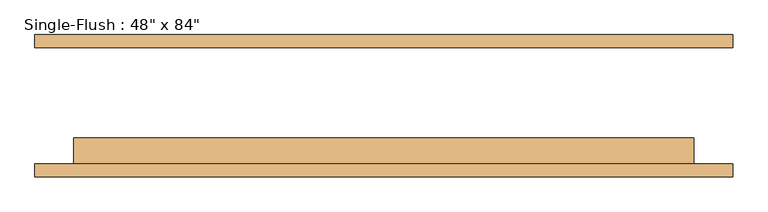
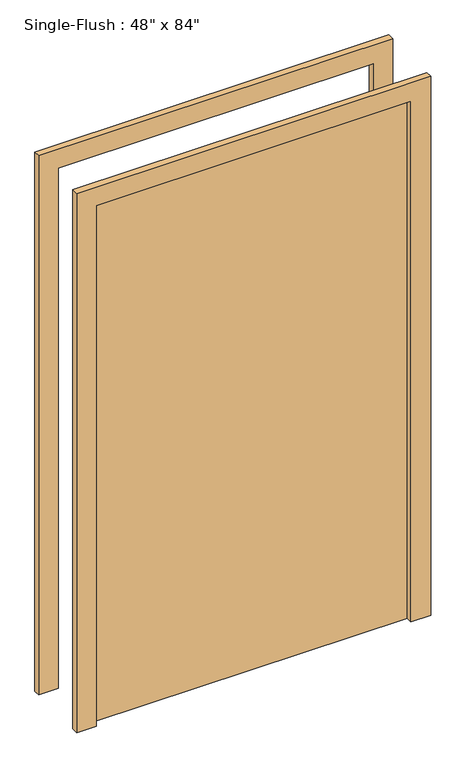
"""IFC4 building model written with IfcOpenShell, lengths in millimetres: door geometry."""

from ifc_helpers import new_model, si_unit, frame, origin, origin_with_axes, place, context, project, spatial, polyline, outline, extrude, source, transform, mapped, element, save


def door_f4c4cdf2(model_context):
    return source(origin(), model_context, "Body", "SweptSolid", [
        extrude(outline(polyline([(2209.8, -685.8), (0.0, -685.8), (0.0, -609.6), (2133.6, -609.6), (2133.6, 609.6), (0.0, 609.6), (0.0, 685.8), (2209.8, 685.8), (2209.8, -685.8)])), frame((0.0, -139.7, 0.0), z_axis=(0.0, 1.0, 0.0), x_axis=(0.0, 0.0, 1.0)), (0.0, 0.0, 1.0), 25.4),
        extrude(outline(polyline([(2209.8, 685.8), (2209.8, -685.8), (0.0, -685.8), (0.0, -609.6), (2133.6, -609.6), (2133.6, 609.6), (0.0, 609.6), (0.0, 685.8), (2209.8, 685.8)])), frame((0.0, 114.3, 0.0), z_axis=(0.0, 1.0, 0.0), x_axis=(0.0, 0.0, 1.0)), (0.0, 0.0, 1.0), 25.4),
        extrude(outline(polyline([(609.6, -63.5), (609.6, -114.3), (-609.6, -114.3), (-609.6, -63.5), (609.6, -63.5)])), origin_with_axes(), (0.0, 0.0, 1.0), 2133.6),
    ])


if __name__ == "__main__":
    model = new_model("IFC4")
    model_context = context("Model", 3, world=origin())
    ifc_project = project(units=[si_unit("LENGTHUNIT", "METRE", prefix="MILLI")], contexts=[model_context])
    site = spatial("IfcSite", under=ifc_project)
    building = spatial("IfcBuilding", under=site)
    placement = place(None, origin())
    door_shape = door_f4c4cdf2(model_context)
    element("IfcDoor", 1, ObjectType="Single-Flush : 48\" x 84\"", at=placement, inside=building, context=model_context, shape_type="MappedRepresentation", body=[
        mapped(door_shape, transform((0.0, 0.0, 0.0), x_axis=(1.0, 0.0, 0.0), y_axis=(0.0, 1.0, 0.0), z_axis=(0.0, 0.0, 1.0))),
    ])
    save(model, "model.ifc")

# Revit data of these elements
# Type "Single-Flush : 48\" x 84\""
#   Type Mark = "5"
#   Construction Type Id = "MDOOR"
#   Assembly Code = "C1020"
#   Analytic Construction = "Metal"
#   Thickness = 0' - 2"
#   Heat Transfer Coefficient (U) = 0.651978 BTU/(h·ft²·°F)
#   Height = 7' - 0"
#   Trim Projection Ext = 0' - 1"
#   Trim Projection Int = 0' - 1"
#   Trim Width = 0' - 3"
#   Width = 4' - 0"
#   Define Thermal Properties by = 1
#   Define Thermal Properties by = 1
#   Door Material = Door - Panel
#   Frame Material = Door - Frame
#   Visual Light Transmittance = 0
#   Solar Heat Gain Coefficient = 0
#   Function = (empty or 0)
#   Wall Closure = (empty or 0)
# Element 1 (IfcDoor, "Single-Flush : 48\" x 84\"")
#   Materials on its faces: "Door - Frame", "Door - Panel"
# Materials
#   "Door - Panel": class "Wood", colour RGB 210 159 95, transparency 0, Cost = 0
#   "Door - Frame": colour RGB 118 70 51, transparency 0, Cost = 0
